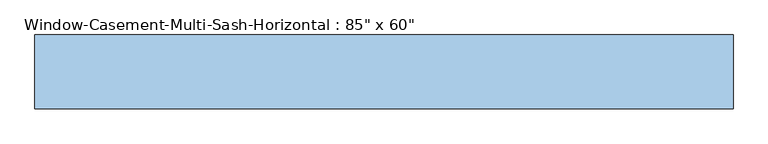
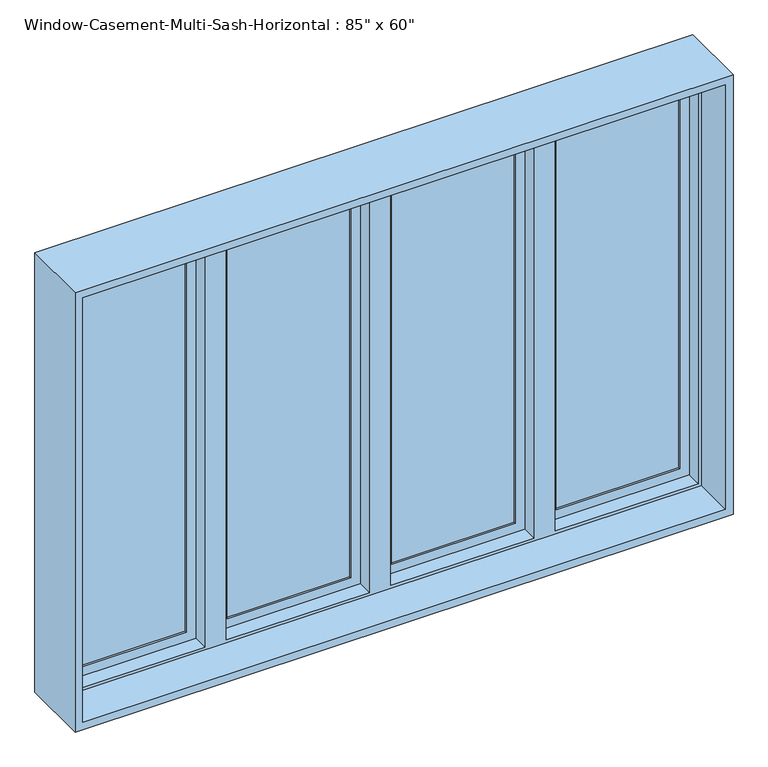
"""IFC4 building model written with IfcOpenShell, lengths in millimetres: window geometry."""

from ifc_helpers import new_model, si_unit, frame, origin, place, context, project, spatial, polyline, outline, extrude, faceted_brep, source, transform, mapped, element, save


def window_a42194c0(model_context):
    return source(origin(), model_context, "Body", "SolidModel", [
        extrude(outline(polyline([(2413.0, 565.15), (939.8, 565.15), (939.8, 1054.1), (2413.0, 1054.1), (2413.0, 565.15)]), holes=[polyline([(2371.1296875, 1012.2296875), (981.6703125, 1012.2296875), (981.6703125, 607.0203125), (2371.1296875, 607.0203125), (2371.1296875, 1012.2296875)])]), frame((0.0, 73.025, 0.0), z_axis=(0.0, 1.0, 0.0), x_axis=(0.0, 0.0, 1.0)), (0.0, 0.0, 1.0), 31.75),
        extrude(outline(polyline([(2413.0, -1054.1), (939.8, -1054.1), (939.8, -565.15), (2413.0, -565.15), (2413.0, -1054.1)]), holes=[polyline([(2371.1296875, -607.0203125), (981.6703125, -607.0203125), (981.6703125, -1012.2296875), (2371.1296875, -1012.2296875), (2371.1296875, -607.0203125)])]), frame((0.0, 73.025, 0.0), z_axis=(0.0, 1.0, 0.0), x_axis=(0.0, 0.0, 1.0)), (0.0, 0.0, 1.0), 31.75),
        extrude(outline(polyline([(-607.0203125, 98.425), (-607.0203125, 92.075), (-1012.2296875, 92.075), (-1012.2296875, 98.425), (-607.0203125, 98.425)])), frame((0.0, 0.0, 981.6703125), z_axis=(0.0, 0.0, 1.0), x_axis=(1.0, 0.0, 0.0)), (0.0, 0.0, 1.0), 1389.459375),
        extrude(outline(polyline([(-607.0203125, 85.725), (-607.0203125, 79.375), (-1012.2296875, 79.375), (-1012.2296875, 85.725), (-607.0203125, 85.725)])), frame((0.0, 0.0, 981.6703125), z_axis=(0.0, 0.0, 1.0), x_axis=(1.0, 0.0, 0.0)), (0.0, 0.0, 1.0), 1389.459375),
        extrude(outline(polyline([(1012.2296875, 98.425), (1012.2296875, 92.075), (607.0203125, 92.075), (607.0203125, 98.425), (1012.2296875, 98.425)])), frame((0.0, 0.0, 981.6703125), z_axis=(0.0, 0.0, 1.0), x_axis=(1.0, 0.0, 0.0)), (0.0, 0.0, 1.0), 1389.459375),
        extrude(outline(polyline([(1012.2296875, 85.725), (1012.2296875, 79.375), (607.0203125, 79.375), (607.0203125, 85.725), (1012.2296875, 85.725)])), frame((0.0, 0.0, 981.6703125), z_axis=(0.0, 0.0, 1.0), x_axis=(1.0, 0.0, 0.0)), (0.0, 0.0, 1.0), 1389.459375),
        extrude(outline(polyline([(-67.2703125, 98.425), (-67.2703125, 92.075), (-472.4796875, 92.075), (-472.4796875, 98.425), (-67.2703125, 98.425)])), frame((0.0, 0.0, 981.6703125), z_axis=(0.0, 0.0, 1.0), x_axis=(1.0, 0.0, 0.0)), (0.0, 0.0, 1.0), 1389.459375),
        extrude(outline(polyline([(-67.2703125, 85.725), (-67.2703125, 79.375), (-472.4796875, 79.375), (-472.4796875, 85.725), (-67.2703125, 85.725)])), frame((0.0, 0.0, 981.6703125), z_axis=(0.0, 0.0, 1.0), x_axis=(1.0, 0.0, 0.0)), (0.0, 0.0, 1.0), 1389.459375),
        extrude(outline(polyline([(472.4796875, 98.425), (472.4796875, 92.075), (67.2703125, 92.075), (67.2703125, 98.425), (472.4796875, 98.425)])), frame((0.0, 0.0, 981.6703125), z_axis=(0.0, 0.0, 1.0), x_axis=(1.0, 0.0, 0.0)), (0.0, 0.0, 1.0), 1389.459375),
        extrude(outline(polyline([(472.4796875, 85.725), (472.4796875, 79.375), (67.2703125, 79.375), (67.2703125, 85.725), (472.4796875, 85.725)])), frame((0.0, 0.0, 981.6703125), z_axis=(0.0, 0.0, 1.0), x_axis=(1.0, 0.0, 0.0)), (0.0, 0.0, 1.0), 1389.459375),
        faceted_brep([(-565.15, 73.025, 2413.0), (-1054.1, 73.025, 2413.0), (-1054.1, 114.3, 2413.0), (1054.1, 114.3, 2413.0), (1054.1, 73.025, 2413.0), (565.15, 73.025, 2413.0), (565.15, 111.125, 2413.0), (514.35, 111.125, 2413.0), (514.35, 73.025, 2413.0), (25.4, 73.025, 2413.0), (25.4, 111.125, 2413.0), (-25.4, 111.125, 2413.0), (-25.4, 73.025, 2413.0), (-514.35, 73.025, 2413.0), (-514.35, 111.125, 2413.0), (-565.15, 111.125, 2413.0), (-1043.9796875, 22.225, 2402.8796875), (-1043.9796875, 73.025, 2402.8796875), (-575.2703125, 73.025, 2402.8796875), (-575.2703125, 22.225, 2402.8796875), (1043.9796875, 73.025, 2402.8796875), (1043.9796875, 22.225, 2402.8796875), (575.2703125, 22.225, 2402.8796875), (575.2703125, 73.025, 2402.8796875), (-504.2296875, 73.025, 2402.8796875), (-35.5203125, 73.025, 2402.8796875), (-35.5203125, 22.225, 2402.8796875), (-504.2296875, 22.225, 2402.8796875), (35.5203125, 73.025, 2402.8796875), (504.2296875, 73.025, 2402.8796875), (504.2296875, 22.225, 2402.8796875), (35.5203125, 22.225, 2402.8796875), (-1054.1, -114.3, 2413.0), (-1054.1, 22.225, 2413.0), (1054.1, 22.225, 2413.0), (1054.1, -114.3, 2413.0), (-1079.5, 114.3, 2438.4), (-1079.5, -114.3, 2438.4), (1079.5, -114.3, 2438.4), (1079.5, 114.3, 2438.4), (1054.1, 114.3, 939.8), (1054.1, 73.025, 939.8), (1043.9796875, 73.025, 949.9203125), (1043.9796875, 22.225, 949.9203125), (1054.1, 22.225, 939.8), (1054.1, -114.3, 939.8), (1079.5, -114.3, 914.4), (1079.5, 114.3, 914.4), (565.15, 73.025, 939.8), (-1054.1, 114.3, 939.8), (-1054.1, 73.025, 939.8), (-565.15, 73.025, 939.8), (-565.15, 111.125, 939.8), (-514.35, 111.125, 939.8), (-514.35, 73.025, 939.8), (-25.4, 73.025, 939.8), (-25.4, 111.125, 939.8), (25.4, 111.125, 939.8), (25.4, 73.025, 939.8), (514.35, 73.025, 939.8), (514.35, 111.125, 939.8), (565.15, 111.125, 939.8), (575.2703125, 73.025, 949.9203125), (575.2703125, 22.225, 949.9203125), (-1043.9796875, 73.025, 949.9203125), (-1043.9796875, 22.225, 949.9203125), (-575.2703125, 22.225, 949.9203125), (-575.2703125, 73.025, 949.9203125), (-35.5203125, 73.025, 949.9203125), (-504.2296875, 73.025, 949.9203125), (-504.2296875, 22.225, 949.9203125), (-35.5203125, 22.225, 949.9203125), (504.2296875, 73.025, 949.9203125), (35.5203125, 73.025, 949.9203125), (35.5203125, 22.225, 949.9203125), (504.2296875, 22.225, 949.9203125), (-1054.1, 22.225, 939.8), (-1054.1, -114.3, 939.8), (-1079.5, -114.3, 914.4), (-1079.5, 114.3, 914.4)], [[[0, 1, 2, 3, 4, 5, 6, 7, 8, 9, 10, 11, 12, 13, 14, 15]], [[16, 17, 18, 19]], [[20, 21, 22, 23]], [[24, 25, 26, 27]], [[28, 29, 30, 31]], [[32, 33, 34, 35]], [[36, 37, 38, 39]], [[4, 3, 40, 41]], [[21, 20, 42, 43]], [[35, 34, 44, 45]], [[39, 38, 46, 47]], [[48, 41, 40, 49, 50, 51, 52, 53, 54, 55, 56, 57, 58, 59, 60, 61]], [[43, 42, 62, 63]], [[64, 65, 66, 67]], [[68, 69, 70, 71]], [[72, 73, 74, 75]], [[45, 44, 76, 77]], [[47, 46, 78, 79]], [[2, 1, 50, 49]], [[4, 41, 48, 5], [20, 23, 62, 42]], [[50, 1, 0, 51], [64, 67, 18, 17]], [[12, 55, 54, 13], [69, 68, 25, 24]], [[8, 59, 58, 9], [73, 72, 29, 28]], [[17, 16, 65, 64]], [[44, 34, 33, 76], [16, 19, 66, 65], [27, 26, 71, 70], [31, 30, 75, 74], [21, 43, 63, 22]], [[33, 32, 77, 76]], [[38, 37, 78, 46], [32, 35, 45, 77]], [[37, 36, 79, 78]], [[36, 39, 47, 79], [3, 2, 49, 40]], [[18, 67, 66, 19]], [[69, 24, 27, 70]], [[53, 14, 13, 54]], [[14, 53, 52, 15]], [[15, 52, 51, 0]], [[25, 68, 71, 26]], [[73, 28, 31, 74]], [[57, 10, 9, 58]], [[10, 57, 56, 11]], [[11, 56, 55, 12]], [[6, 61, 60, 7]], [[7, 60, 59, 8]], [[29, 72, 75, 30]], [[62, 23, 22, 63]], [[61, 6, 5, 48]]]),
        extrude(outline(polyline([(2413.0, 25.4), (939.8, 25.4), (939.8, 514.35), (2413.0, 514.35), (2413.0, 25.4)]), holes=[polyline([(2371.1296875, 472.4796875), (981.6703125, 472.4796875), (981.6703125, 67.2703125), (2371.1296875, 67.2703125), (2371.1296875, 472.4796875)])]), frame((0.0, 73.025, 0.0), z_axis=(0.0, 1.0, 0.0), x_axis=(0.0, 0.0, 1.0)), (0.0, 0.0, 1.0), 31.75),
        extrude(outline(polyline([(2413.0, -514.35), (939.8, -514.35), (939.8, -25.4), (2413.0, -25.4), (2413.0, -514.35)]), holes=[polyline([(2371.1296875, -67.2703125), (981.6703125, -67.2703125), (981.6703125, -472.4796875), (2371.1296875, -472.4796875), (2371.1296875, -67.2703125)])]), frame((0.0, 73.025, 0.0), z_axis=(0.0, 1.0, 0.0), x_axis=(0.0, 0.0, 1.0)), (0.0, 0.0, 1.0), 31.75),
    ])


if __name__ == "__main__":
    model = new_model("IFC4")
    model_context = context("Model", 3, world=origin())
    ifc_project = project(units=[si_unit("LENGTHUNIT", "METRE", prefix="MILLI")], contexts=[model_context])
    site = spatial("IfcSite", under=ifc_project)
    building = spatial("IfcBuilding", under=site)
    placement = place(None, origin())
    window_shape = window_a42194c0(model_context)
    element("IfcWindow", 1, ObjectType="Window-Casement-Multi-Sash-Horizontal : 85\" x 60\"", at=placement, inside=building, context=model_context, shape_type="MappedRepresentation", body=[
        mapped(window_shape, transform((0.0, 0.0, 0.0), x_axis=(1.0, 0.0, 0.0), y_axis=(0.0, 1.0, 0.0), z_axis=(0.0, 0.0, 1.0))),
    ])
    save(model, "model.ifc")

# Revit data of these elements
# Type "Window-Casement-Multi-Sash-Horizontal : 85\" x 60\""
#   Type Mark = "24"
#   Fire Rating = "0.5h"
#   Assembly Code = "B2020100"
#   Analytic Construction = "Double glazing - domestic"
#   Window Inset [instance default] = 0' - 0 5/8"
#   Wall Thickness [instance default] = 0' - 6"
#   Visual Light Transmittance = 0.81
#   Thermal Resistance (R) = 1.8146 (h·ft²·°F)/BTU
#   Solar Heat Gain Coefficient = 0.76
#   Rough Width = 7' - 1 1/2"
#   Rough Height = 5' - 0 1/2"
#   Open Window Width = 1' - 9 1/4"
#   Heat Transfer Coefficient (U) = 0.5511 BTU/(h·ft²·°F)
#   Height = 5' - 0"
#   Frame Gap 3 [instance default] = 0' - 1 83/128"
#   Frame Gap 2 [instance default] = 0' - 0 5/8"
#   Frame Gap 1 = 0' - 1 51/128"
#   Default Sill Height = 3' - 0"
#   Width = 7' - 1"
#   Frame Material = Metal - Aluminum
#   Glass Panel Material = Glass
#   Wall Closure = (empty or 0)
# Element 1 (IfcWindow, "Window-Casement-Multi-Sash-Horizontal : 85\" x 60\"")
#   Wall Thickness = 0' - 9"
#   Materials on its faces: "Metal - Aluminum", "Glass"
# Materials
#   "Metal - Aluminum": class "Metal", colour RGB 247 247 247, transparency 0
#   "Glass": class "Glass", colour RGB 0 128 192, transparency 0.75, Description = "Soda Lime Glass", Cost = 0
